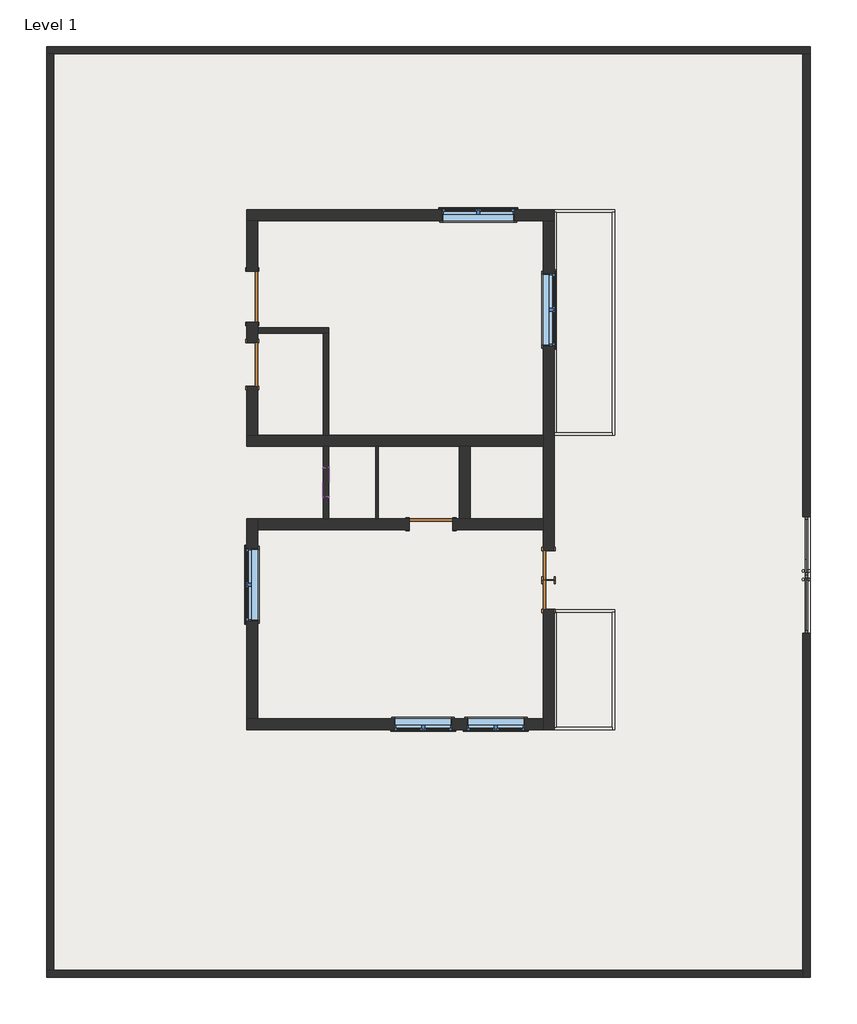
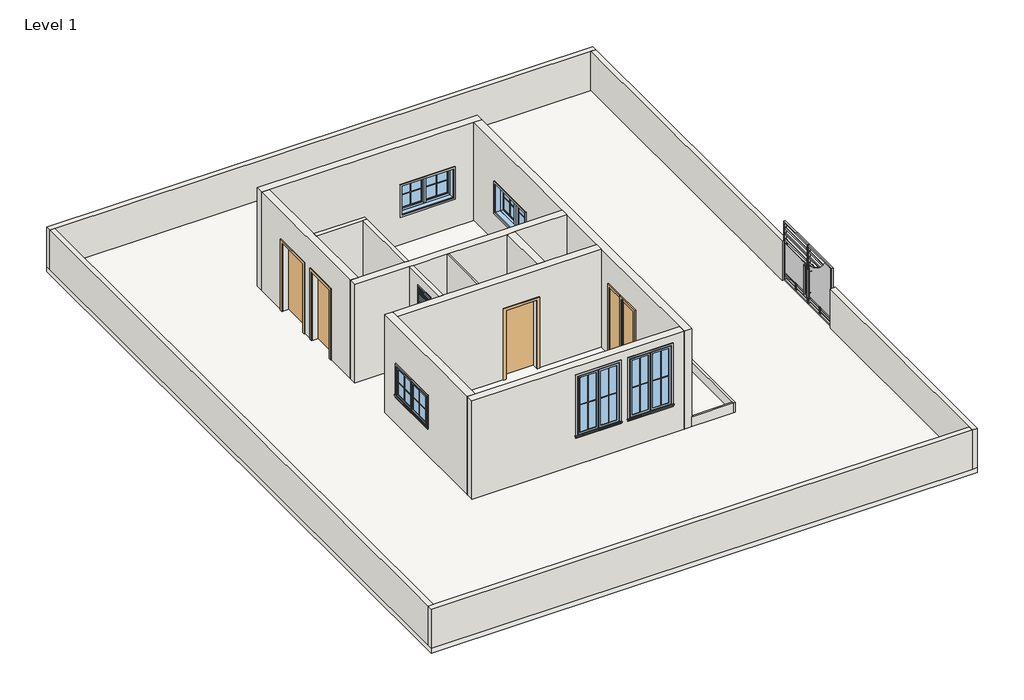
# One storey: 25 walls, 21 proxies, 6 windows, 5 doors, 1 slab.
"""IFC4 building model written with IfcOpenShell, lengths in millimetres."""

from ifc_helpers import new_model, si_unit, frame, origin, origin_with_axes, place, context, project, spatial, polyline, outline, extrude, faceted_brep, transform, mapped, element, save
from components import generic_models_113f6068, muntin_pattern_2x2_muntin_pattern_2x2_9352d081, muntin_pattern_2x2_muntin_pattern_2x2_5c2cbe28, muntin_pattern_2x2_muntin_pattern_2x2_2b4d9f72, muntin_pattern_2x2_muntin_pattern_2x2_ef995ed3, trim_window_exterior_flat_with_sill_979bde60, trim_window_exterior_flat_with_sill_b7e4d11c, trim_window_interior_flat_picture_frame_7883d11b, trim_window_interior_flat_picture_frame_936b8d2a, single_flush_door_2_0d3b4037, single_flush_door_2_4a3212df, door_a90ba1ad, door_0ca8825f, door_9d399b00, window_casement_double_c1d95f0f, window_casement_double_wall_4_6ca1769e, window_d39e7ecb

model = new_model("IFC4")

# Units and contexts
model_context = context("Model", 3, world=origin())
ifc_project = project(units=[si_unit("LENGTHUNIT", "METRE", prefix="MILLI")], contexts=[model_context])

# Site, building, storey
site = spatial("IfcSite", under=ifc_project)
building = spatial("IfcBuilding", under=site)
storey = spatial("IfcBuildingStorey", under=building, Name="Level 1", Elevation=0.0)

# Proxies
placement = place(None, origin())
generic_models_shape = generic_models_113f6068(model_context)
element("IfcBuildingElementProxy", 1, Name="Generic Models", at=placement, inside=storey, context=model_context, shape_type="MappedRepresentation", body=[
    mapped(generic_models_shape, transform((6909.9576308, -2125.2492544, 0.0), x_axis=(0.0, 1.0, 0.0), y_axis=(-1.0, 0.0, 0.0), z_axis=(0.0, 0.0, 1.0))),
])
muntin_pattern_2x2_muntin_pattern_2x2_shape = muntin_pattern_2x2_muntin_pattern_2x2_9352d081(model_context)
element("IfcBuildingElementProxy", 2, Name="Muntin Pattern_2x2 : Muntin Pattern_2x2", ObjectType="Muntin Pattern_2x2 : Muntin Pattern_2x2", at=placement, inside=storey, context=model_context, shape_type="MappedRepresentation", body=[
    mapped(muntin_pattern_2x2_muntin_pattern_2x2_shape, transform((-4785.3510342, -2707.8617544, 984.25), x_axis=(0.0, 1.0, 0.0), y_axis=(-1.0, 0.0, 0.0), z_axis=(0.0, 0.0, 1.0))),
])
element("IfcBuildingElementProxy", 3, Name="Muntin Pattern_2x2 : Muntin Pattern_2x2", ObjectType="Muntin Pattern_2x2 : Muntin Pattern_2x2", at=placement, inside=storey, context=model_context, shape_type="MappedRepresentation", body=[
    mapped(muntin_pattern_2x2_muntin_pattern_2x2_shape, transform((1634.4989658, 3816.7632456, 984.25), x_axis=(0.0, -1.0, 0.0), y_axis=(1.0, 0.0, 0.0), z_axis=(0.0, 0.0, 1.0))),
])
element("IfcBuildingElementProxy", 4, Name="Muntin Pattern_2x2 : Muntin Pattern_2x2", ObjectType="Muntin Pattern_2x2 : Muntin Pattern_2x2", at=placement, inside=storey, context=model_context, shape_type="MappedRepresentation", body=[
    mapped(muntin_pattern_2x2_muntin_pattern_2x2_shape, transform((-322.8885342, 5523.3257456, 984.25), x_axis=(1.0, 0.0, 0.0), y_axis=(0.0, 1.0, 0.0), z_axis=(0.0, 0.0, 1.0))),
])
muntin_pattern_2x2_muntin_pattern_2x2_2_shape = muntin_pattern_2x2_muntin_pattern_2x2_5c2cbe28(model_context)
element("IfcBuildingElementProxy", 5, Name="Muntin Pattern_2x2 : Muntin Pattern_2x2", ObjectType="Muntin Pattern_2x2 : Muntin Pattern_2x2", at=placement, inside=storey, context=model_context, shape_type="MappedRepresentation", body=[
    mapped(muntin_pattern_2x2_muntin_pattern_2x2_2_shape, transform((-4785.3510342, -1949.0367544, 984.25), x_axis=(0.0, -1.0, 0.0), y_axis=(1.0, 0.0, 0.0), z_axis=(0.0, 0.0, 1.0))),
])
element("IfcBuildingElementProxy", 6, Name="Muntin Pattern_2x2 : Muntin Pattern_2x2", ObjectType="Muntin Pattern_2x2 : Muntin Pattern_2x2", at=placement, inside=storey, context=model_context, shape_type="MappedRepresentation", body=[
    mapped(muntin_pattern_2x2_muntin_pattern_2x2_2_shape, transform((1634.4989658, 3057.9382456, 984.25), x_axis=(0.0, 1.0, 0.0), y_axis=(-1.0, 0.0, 0.0), z_axis=(0.0, 0.0, 1.0))),
])
element("IfcBuildingElementProxy", 7, Name="Muntin Pattern_2x2 : Muntin Pattern_2x2", ObjectType="Muntin Pattern_2x2 : Muntin Pattern_2x2", at=placement, inside=storey, context=model_context, shape_type="MappedRepresentation", body=[
    mapped(muntin_pattern_2x2_muntin_pattern_2x2_2_shape, transform((435.9364658, 5523.3257456, 984.25), x_axis=(-1.0, 0.0, 0.0), y_axis=(0.0, -1.0, 0.0), z_axis=(0.0, 0.0, 1.0))),
])
muntin_pattern_2x2_muntin_pattern_2x2_3_shape = muntin_pattern_2x2_muntin_pattern_2x2_2b4d9f72(model_context)
element("IfcBuildingElementProxy", 8, Name="Muntin Pattern_2x2 : Muntin Pattern_2x2", ObjectType="Muntin Pattern_2x2 : Muntin Pattern_2x2", at=placement, inside=storey, context=model_context, shape_type="MappedRepresentation", body=[
    mapped(muntin_pattern_2x2_muntin_pattern_2x2_3_shape, transform((-795.9635342, -5354.2242544, 984.25), x_axis=(-1.0, 0.0, 0.0), y_axis=(0.0, -1.0, 0.0), z_axis=(0.0, 0.0, 1.0))),
])
element("IfcBuildingElementProxy", 9, Name="Muntin Pattern_2x2 : Muntin Pattern_2x2", ObjectType="Muntin Pattern_2x2 : Muntin Pattern_2x2", at=placement, inside=storey, context=model_context, shape_type="MappedRepresentation", body=[
    mapped(muntin_pattern_2x2_muntin_pattern_2x2_3_shape, transform((728.0364658, -5354.2242544, 984.25), x_axis=(-1.0, 0.0, 0.0), y_axis=(0.0, -1.0, 0.0), z_axis=(0.0, 0.0, 1.0))),
])
muntin_pattern_2x2_muntin_pattern_2x2_4_shape = muntin_pattern_2x2_muntin_pattern_2x2_ef995ed3(model_context)
element("IfcBuildingElementProxy", 10, Name="Muntin Pattern_2x2 : Muntin Pattern_2x2", ObjectType="Muntin Pattern_2x2 : Muntin Pattern_2x2", at=placement, inside=storey, context=model_context, shape_type="MappedRepresentation", body=[
    mapped(muntin_pattern_2x2_muntin_pattern_2x2_4_shape, transform((-1402.3885342, -5354.2242544, 984.25), x_axis=(1.0, 0.0, 0.0), y_axis=(0.0, 1.0, 0.0), z_axis=(0.0, 0.0, 1.0))),
])
element("IfcBuildingElementProxy", 11, Name="Muntin Pattern_2x2 : Muntin Pattern_2x2", ObjectType="Muntin Pattern_2x2 : Muntin Pattern_2x2", at=placement, inside=storey, context=model_context, shape_type="MappedRepresentation", body=[
    mapped(muntin_pattern_2x2_muntin_pattern_2x2_4_shape, transform((121.6114658, -5354.2242544, 984.25), x_axis=(1.0, 0.0, 0.0), y_axis=(0.0, 1.0, 0.0), z_axis=(0.0, 0.0, 1.0))),
])
trim_window_exterior_flat_with_sill_shape = trim_window_exterior_flat_with_sill_979bde60(model_context)
element("IfcBuildingElementProxy", 12, Name="Trim-Window-Exterior-Flat : with Sill", ObjectType="Trim-Window-Exterior-Flat : with Sill", at=placement, inside=storey, context=model_context, shape_type="MappedRepresentation", body=[
    mapped(trim_window_exterior_flat_with_sill_shape, transform((-4794.8760342, -2328.4492544, 1828.8), x_axis=(0.0, -1.0, 0.0), y_axis=(0.0, 0.0, 1.0), z_axis=(-1.0, 0.0, 0.0))),
])
element("IfcBuildingElementProxy", 13, Name="Trim-Window-Exterior-Flat : with Sill", ObjectType="Trim-Window-Exterior-Flat : with Sill", at=placement, inside=storey, context=model_context, shape_type="MappedRepresentation", body=[
    mapped(trim_window_exterior_flat_with_sill_shape, transform((1644.0239658, 3437.3507456, 1828.8), x_axis=(0.0, 1.0, 0.0), y_axis=(0.0, 0.0, 1.0), z_axis=(1.0, 0.0, 0.0))),
])
element("IfcBuildingElementProxy", 14, Name="Trim-Window-Exterior-Flat : with Sill", ObjectType="Trim-Window-Exterior-Flat : with Sill", at=placement, inside=storey, context=model_context, shape_type="MappedRepresentation", body=[
    mapped(trim_window_exterior_flat_with_sill_shape, transform((56.5239658, 5532.8507456, 1828.8), x_axis=(-1.0, 0.0, 0.0), y_axis=(0.0, 0.0, 1.0), z_axis=(0.0, 1.0, 0.0))),
])
trim_window_exterior_flat_with_sill_2_shape = trim_window_exterior_flat_with_sill_b7e4d11c(model_context)
element("IfcBuildingElementProxy", 15, Name="Trim-Window-Exterior-Flat : with Sill", ObjectType="Trim-Window-Exterior-Flat : with Sill", at=placement, inside=storey, context=model_context, shape_type="MappedRepresentation", body=[
    mapped(trim_window_exterior_flat_with_sill_2_shape, transform((-1099.1760342, -5363.7492544, 2743.2), x_axis=(1.0, 0.0, 0.0), y_axis=(0.0, 0.0, 1.0), z_axis=(0.0, -1.0, 0.0))),
])
element("IfcBuildingElementProxy", 16, Name="Trim-Window-Exterior-Flat : with Sill", ObjectType="Trim-Window-Exterior-Flat : with Sill", at=placement, inside=storey, context=model_context, shape_type="MappedRepresentation", body=[
    mapped(trim_window_exterior_flat_with_sill_2_shape, transform((424.8239658, -5363.7492544, 2743.2), x_axis=(1.0, 0.0, 0.0), y_axis=(0.0, 0.0, 1.0), z_axis=(0.0, -1.0, 0.0))),
])
trim_window_interior_flat_picture_frame_shape = trim_window_interior_flat_picture_frame_7883d11b(model_context)
element("IfcBuildingElementProxy", 17, Name="Trim-Window-Interior-Flat : Picture Frame", ObjectType="Trim-Window-Interior-Flat : Picture Frame", at=placement, inside=storey, context=model_context, shape_type="MappedRepresentation", body=[
    mapped(trim_window_interior_flat_picture_frame_shape, transform((-4566.2760342, -2328.4492544, 1828.8), x_axis=(0.0, 1.0, 0.0), y_axis=(0.0, 0.0, 1.0), z_axis=(1.0, 0.0, 0.0))),
])
element("IfcBuildingElementProxy", 18, Name="Trim-Window-Interior-Flat : Picture Frame", ObjectType="Trim-Window-Interior-Flat : Picture Frame", at=placement, inside=storey, context=model_context, shape_type="MappedRepresentation", body=[
    mapped(trim_window_interior_flat_picture_frame_shape, transform((1415.4239658, 3437.3507456, 1828.8), x_axis=(0.0, -1.0, 0.0), y_axis=(0.0, 0.0, 1.0), z_axis=(-1.0, 0.0, 0.0))),
])
element("IfcBuildingElementProxy", 19, Name="Trim-Window-Interior-Flat : Picture Frame", ObjectType="Trim-Window-Interior-Flat : Picture Frame", at=placement, inside=storey, context=model_context, shape_type="MappedRepresentation", body=[
    mapped(trim_window_interior_flat_picture_frame_shape, transform((56.5239658, 5304.2507456, 1828.8), x_axis=(1.0, 0.0, 0.0), y_axis=(0.0, 0.0, 1.0), z_axis=(0.0, -1.0, 0.0))),
])
trim_window_interior_flat_picture_frame_2_shape = trim_window_interior_flat_picture_frame_936b8d2a(model_context)
element("IfcBuildingElementProxy", 20, Name="Trim-Window-Interior-Flat : Picture Frame", ObjectType="Trim-Window-Interior-Flat : Picture Frame", at=placement, inside=storey, context=model_context, shape_type="MappedRepresentation", body=[
    mapped(trim_window_interior_flat_picture_frame_2_shape, transform((-1099.1760342, -5135.1492544, 2743.2), x_axis=(-1.0, 0.0, 0.0), y_axis=(0.0, 0.0, 1.0), z_axis=(0.0, 1.0, 0.0))),
])
element("IfcBuildingElementProxy", 21, Name="Trim-Window-Interior-Flat : Picture Frame", ObjectType="Trim-Window-Interior-Flat : Picture Frame", at=placement, inside=storey, context=model_context, shape_type="MappedRepresentation", body=[
    mapped(trim_window_interior_flat_picture_frame_2_shape, transform((424.8239658, -5135.1492544, 2743.2), x_axis=(-1.0, 0.0, 0.0), y_axis=(0.0, 0.0, 1.0), z_axis=(0.0, 1.0, 0.0))),
])

# Doors
single_flush_door_2_shape = single_flush_door_2_0d3b4037(model_context)
element("IfcDoor", 22, ObjectType="Single-Flush : door 2'", at=placement, inside=storey, context=model_context, shape_type="MappedRepresentation", body=[
    mapped(single_flush_door_2_shape, transform((1529.7239658, -1922.0492544, 0.0), x_axis=(0.0, 1.0, 0.0), y_axis=(-1.0, 0.0, 0.0), z_axis=(0.0, 0.0, 1.0))),
])
single_flush_door_2_2_shape = single_flush_door_2_4a3212df(model_context)
element("IfcDoor", 23, ObjectType="Single-Flush : door 2'", at=placement, inside=storey, context=model_context, shape_type="MappedRepresentation", body=[
    mapped(single_flush_door_2_2_shape, transform((1529.7239658, -2537.9992544, 0.0), x_axis=(0.0, -1.0, 0.0), y_axis=(1.0, 0.0, 0.0), z_axis=(0.0, 0.0, 1.0))),
])
door_shape = door_a90ba1ad(model_context)
element("IfcDoor", 24, ObjectType="Single-Flush : door 2'6\"", at=placement, inside=storey, context=model_context, shape_type="MappedRepresentation", body=[
    mapped(door_shape, transform((-4680.5760342, 2288.0007456, 0.0), x_axis=(0.0, 1.0, 0.0), y_axis=(-1.0, 0.0, 0.0), z_axis=(0.0, 0.0, 1.0))),
])
door_2_shape = door_0ca8825f(model_context)
element("IfcDoor", 25, ObjectType="Single-Flush : door 2'6\"", at=placement, inside=storey, context=model_context, shape_type="MappedRepresentation", body=[
    mapped(door_2_shape, transform((-934.0760342, -1058.4492544, 0.0), x_axis=(1.0, 0.0, 0.0), y_axis=(0.0, 1.0, 0.0), z_axis=(0.0, 0.0, 1.0))),
])
door_3_shape = door_9d399b00(model_context)
element("IfcDoor", 26, ObjectType="Single-Flush : door 3'6\"", at=placement, inside=storey, context=model_context, shape_type="MappedRepresentation", body=[
    mapped(door_3_shape, transform((-4680.5760342, 3710.4007456, 0.0), x_axis=(0.0, -1.0, 0.0), y_axis=(1.0, 0.0, 0.0), z_axis=(0.0, 0.0, 1.0))),
])

# Slab
element("IfcSlab", 27, ObjectType="floor 6\"", at=placement, inside=storey, context=model_context, shape_type="SweptSolid", body=[
    extrude(outline(polyline([(7011.5576308, 8950.777895), (7011.5576308, -10556.422105), (-8990.4423692, -10556.422105), (-8990.4423692, 8950.777895), (7011.5576308, 8950.777895)])), frame((0.0, 0.0, -152.4), z_axis=(0.0, 0.0, 1.0), x_axis=(1.0, 0.0, 0.0)), (0.0, 0.0, 1.0), 152.4),
])

# Walls
element("IfcWall", 28, at=placement, inside=storey, context=model_context, shape_type="Brep", body=[
    faceted_brep([(-8990.4423692, 8798.377895, 0.0), (-8838.0423692, 8798.377895, 0.0), (6859.1576308, 8798.377895, 0.0), (7011.5576308, 8798.377895, 0.0), (7011.5576308, 8798.377895, 1219.2), (6859.1576308, 8798.377895, 1219.2), (-8838.0423692, 8798.377895, 1219.2), (-8990.4423692, 8798.377895, 1219.2), (-8990.4423692, 8950.777895, 0.0), (-8990.4423692, 8950.777895, 1219.2), (7011.5576308, 8950.777895, 1219.2), (7011.5576308, 8950.777895, 0.0)], [[[0, 1, 2, 3, 4, 5, 6, 7]], [[8, 9, 10, 11]], [[3, 2, 1, 0, 8, 11]], [[7, 6, 5, 4, 10, 9]], [[4, 3, 11, 10]], [[0, 7, 9, 8]]]),
])
element("IfcWall", 29, at=placement, inside=storey, context=model_context, shape_type="SweptSolid", body=[
    extrude(outline(polyline([(6859.1576308, -906.0492544), (6859.1576308, 8798.377895), (7011.5576308, 8798.377895), (7011.5576308, -906.0492544), (6859.1576308, -906.0492544)])), origin_with_axes(), (0.0, 0.0, 1.0), 1219.2),
])
element("IfcWall", 30, at=placement, inside=storey, context=model_context, shape_type="Brep", body=[
    faceted_brep([(6859.1576308, -10404.022105, 0.0), (-8838.0423692, -10404.022105, 0.0), (-8990.4423692, -10404.022105, 0.0), (-8990.4423692, -10404.022105, 1219.2), (-8838.0423692, -10404.022105, 1219.2), (6859.1576308, -10404.022105, 1219.2), (6859.1576308, -10556.422105, 0.0), (6859.1576308, -10556.422105, 1219.2), (-8990.4423692, -10556.422105, 1219.2), (-8990.4423692, -10556.422105, 0.0)], [[[0, 1, 2, 3, 4, 5]], [[6, 7, 8, 9]], [[2, 1, 0, 6, 9]], [[5, 4, 3, 8, 7]], [[0, 5, 7, 6]], [[3, 2, 9, 8]]]),
])
element("IfcWall", 31, at=placement, inside=storey, context=model_context, shape_type="SweptSolid", body=[
    extrude(outline(polyline([(-8838.0423692, 8798.377895), (-8838.0423692, -10404.022105), (-8990.4423692, -10404.022105), (-8990.4423692, 8798.377895), (-8838.0423692, 8798.377895)])), origin_with_axes(), (0.0, 0.0, 1.0), 1219.2),
])
element("IfcWall", 32, at=placement, inside=storey, context=model_context, shape_type="Brep", body=[
    faceted_brep([(6859.1576308, -3344.4492544, 0.0), (6859.1576308, -10404.022105, 0.0), (6859.1576308, -10556.422105, 0.0), (6859.1576308, -10556.422105, 1219.2), (6859.1576308, -10404.022105, 1219.2), (6859.1576308, -3344.4492544, 1219.2), (7011.5576308, -3344.4492544, 0.0), (7011.5576308, -3344.4492544, 1219.2), (7011.5576308, -10556.422105, 1219.2), (7011.5576308, -10556.422105, 0.0)], [[[0, 1, 2, 3, 4, 5]], [[6, 7, 8, 9]], [[2, 1, 0, 6, 9]], [[5, 4, 3, 8, 7]], [[0, 5, 7, 6]], [[3, 2, 9, 8]]]),
])
element("IfcWall", 33, ObjectType="wall 2\"", at=placement, inside=storey, context=model_context, shape_type="SweptSolid", body=[
    extrude(outline(polyline([(-2089.7760342, -944.1492544), (-2089.7760342, 579.8507456), (-2038.9760342, 579.8507456), (-2038.9760342, -944.1492544), (-2089.7760342, -944.1492544)])), origin_with_axes(), (0.0, 0.0, 1.0), 3048.0),
])
element("IfcWall", 34, ObjectType="wall 2\"", at=placement, inside=storey, context=model_context, shape_type="Brep", body=[
    faceted_brep([(1644.0239658, 5482.0507456, 0.0), (1694.8239658, 5482.0507456, 0.0), (2863.2239658, 5482.0507456, 0.0), (2914.0239658, 5482.0507456, 0.0), (2914.0239658, 5482.0507456, 304.8), (2863.2239658, 5482.0507456, 304.8), (1694.8239658, 5482.0507456, 304.8), (1644.0239658, 5482.0507456, 304.8), (1644.0239658, 5532.8507456, 0.0), (1644.0239658, 5532.8507456, 304.8), (2914.0239658, 5532.8507456, 304.8), (2914.0239658, 5532.8507456, 0.0)], [[[0, 1, 2, 3, 4, 5, 6, 7]], [[8, 9, 10, 11]], [[3, 2, 1, 0, 8, 11]], [[7, 6, 5, 4, 10, 9]], [[0, 7, 9, 8]], [[4, 3, 11, 10]]]),
])
element("IfcWall", 35, ObjectType="wall 2\"", at=placement, inside=storey, context=model_context, shape_type="Brep", body=[
    faceted_brep([(2863.2239658, 5482.0507456, 0.0), (2863.2239658, 859.2507456, 0.0), (2863.2239658, 808.4507456, 0.0), (2863.2239658, 808.4507456, 304.8), (2863.2239658, 859.2507456, 304.8), (2863.2239658, 5482.0507456, 304.8), (2914.0239658, 5482.0507456, 0.0), (2914.0239658, 5482.0507456, 304.8), (2914.0239658, 808.4507456, 304.8), (2914.0239658, 808.4507456, 0.0)], [[[0, 1, 2, 3, 4, 5]], [[6, 7, 8, 9]], [[2, 1, 0, 6, 9]], [[5, 4, 3, 8, 7]], [[0, 5, 7, 6]], [[3, 2, 9, 8]]]),
])
element("IfcWall", 36, ObjectType="wall 2\"", at=placement, inside=storey, context=model_context, shape_type="Brep", body=[
    faceted_brep([(2863.2239658, 859.2507456, 0.0), (1694.8239658, 859.2507456, 0.0), (1644.0239658, 859.2507456, 0.0), (1644.0239658, 859.2507456, 304.8), (1694.8239658, 859.2507456, 304.8), (2863.2239658, 859.2507456, 304.8), (2863.2239658, 808.4507456, 0.0), (2863.2239658, 808.4507456, 304.8), (1644.0239658, 808.4507456, 304.8), (1644.0239658, 808.4507456, 0.0)], [[[0, 1, 2, 3, 4, 5]], [[6, 7, 8, 9]], [[2, 1, 0, 6, 9]], [[5, 4, 3, 8, 7]], [[0, 5, 7, 6]], [[3, 2, 9, 8]]]),
])
element("IfcWall", 37, ObjectType="wall 2\"", at=placement, inside=storey, context=model_context, shape_type="Brep", body=[
    faceted_brep([(1694.8239658, 859.2507456, 0.0), (1694.8239658, 5482.0507456, 0.0), (1694.8239658, 5482.0507456, 304.8), (1694.8239658, 859.2507456, 304.8), (1644.0239658, 859.2507456, 0.0), (1644.0239658, 859.2507456, 304.8), (1644.0239658, 5482.0507456, 304.8), (1644.0239658, 5482.0507456, 0.0), (1644.0239658, 5304.2507456, 0.0)], [[[0, 1, 2, 3]], [[4, 5, 6, 7, 8]], [[1, 0, 4, 8, 7]], [[3, 2, 6, 5]], [[2, 1, 7, 6]], [[0, 3, 5, 4]]]),
])
element("IfcWall", 38, ObjectType="wall 2\"", at=placement, inside=storey, context=model_context, shape_type="Brep", body=[
    faceted_brep([(1644.0239658, -2899.9492544, 0.0), (1694.8239658, -2899.9492544, 0.0), (2863.2239658, -2899.9492544, 0.0), (2914.0239658, -2899.9492544, 0.0), (2914.0239658, -2899.9492544, 304.8), (2863.2239658, -2899.9492544, 304.8), (1694.8239658, -2899.9492544, 304.8), (1644.0239658, -2899.9492544, 304.8), (1644.0239658, -2849.1492544, 0.0), (1644.0239658, -2849.1492544, 304.8), (2914.0239658, -2849.1492544, 304.8), (2914.0239658, -2849.1492544, 0.0)], [[[0, 1, 2, 3, 4, 5, 6, 7]], [[8, 9, 10, 11]], [[3, 2, 1, 0, 8, 11]], [[7, 6, 5, 4, 10, 9]], [[0, 7, 9, 8]], [[4, 3, 11, 10]]]),
])
element("IfcWall", 39, ObjectType="wall 2\"", at=placement, inside=storey, context=model_context, shape_type="Brep", body=[
    faceted_brep([(2863.2239658, -2899.9492544, 0.0), (2863.2239658, -5312.9492544, 0.0), (2863.2239658, -5363.7492544, 0.0), (2863.2239658, -5363.7492544, 304.8), (2863.2239658, -5312.9492544, 304.8), (2863.2239658, -2899.9492544, 304.8), (2914.0239658, -2899.9492544, 0.0), (2914.0239658, -2899.9492544, 304.8), (2914.0239658, -5363.7492544, 304.8), (2914.0239658, -5363.7492544, 0.0)], [[[0, 1, 2, 3, 4, 5]], [[6, 7, 8, 9]], [[2, 1, 0, 6, 9]], [[5, 4, 3, 8, 7]], [[0, 5, 7, 6]], [[3, 2, 9, 8]]]),
])
element("IfcWall", 40, ObjectType="wall 2\"", at=placement, inside=storey, context=model_context, shape_type="Brep", body=[
    faceted_brep([(2863.2239658, -5312.9492544, 0.0), (1694.8239658, -5312.9492544, 0.0), (1644.0239658, -5312.9492544, 0.0), (1644.0239658, -5312.9492544, 304.8), (1694.8239658, -5312.9492544, 304.8), (2863.2239658, -5312.9492544, 304.8), (2863.2239658, -5363.7492544, 0.0), (2863.2239658, -5363.7492544, 304.8), (1644.0239658, -5363.7492544, 304.8), (1644.0239658, -5363.7492544, 0.0)], [[[0, 1, 2, 3, 4, 5]], [[6, 7, 8, 9]], [[2, 1, 0, 6, 9]], [[5, 4, 3, 8, 7]], [[0, 5, 7, 6]], [[3, 2, 9, 8]]]),
])
element("IfcWall", 41, ObjectType="wall 2\"", at=placement, inside=storey, context=model_context, shape_type="SweptSolid", body=[
    extrude(outline(polyline([(1694.8239658, -2899.9492544), (1694.8239658, -5312.9492544), (1644.0239658, -5312.9492544), (1644.0239658, -2899.9492544), (1694.8239658, -2899.9492544)])), origin_with_axes(), (0.0, 0.0, 1.0), 304.8),
])
element("IfcWall", 42, ObjectType="wall 4.5\"", at=placement, inside=storey, context=model_context, shape_type="Brep", body=[
    faceted_brep([(-4566.2760342, 2942.0507456, 0.0), (-3194.6760342, 2942.0507456, 0.0), (-3080.3760342, 2942.0507456, 0.0), (-3080.3760342, 2942.0507456, 3048.0), (-3194.6760342, 2942.0507456, 3048.0), (-4566.2760342, 2942.0507456, 3048.0), (-4566.2760342, 3056.3507456, 0.0), (-4566.2760342, 3056.3507456, 3048.0), (-3080.3760342, 3056.3507456, 3048.0), (-3080.3760342, 3056.3507456, 0.0)], [[[0, 1, 2, 3, 4, 5]], [[6, 7, 8, 9]], [[2, 1, 0, 6, 9]], [[0, 5, 7, 6]], [[3, 2, 9, 8]], [[5, 4, 3, 8, 7]]]),
])
element("IfcWall", 43, ObjectType="wall 4.5\"", at=placement, inside=storey, context=model_context, shape_type="SweptSolid", body=[
    extrude(outline(polyline([(-3194.6760342, 808.4507456), (-3194.6760342, 2942.0507456), (-3080.3760342, 2942.0507456), (-3080.3760342, 808.4507456), (-3194.6760342, 808.4507456)])), origin_with_axes(), (0.0, 0.0, 1.0), 3048.0),
])
element("IfcWall", 44, ObjectType="wall 4.5\"", at=placement, inside=storey, context=model_context, shape_type="SweptSolid", body=[
    extrude(outline(polyline([(579.8507456, 0.0), (-944.1492544, 0.0), (-944.1492544, 3048.0), (579.8507456, 3048.0), (579.8507456, 0.0)]), holes=[polyline([(-486.9492544, 2743.2), (-486.9492544, 2133.6), (122.6507456, 2133.6), (122.6507456, 2743.2), (-486.9492544, 2743.2)])]), frame((-3194.6760342, 0.0, 0.0), z_axis=(1.0, 0.0, 0.0), x_axis=(0.0, 1.0, 0.0)), (0.0, 0.0, 1.0), 114.3),
])
element("IfcWall", 45, ObjectType="wall 9\"", at=placement, inside=storey, context=model_context, shape_type="Brep", body=[
    faceted_brep([(-4794.8760342, 5304.2507456, 0.0), (-4566.2760342, 5304.2507456, 0.0), (1415.4239658, 5304.2507456, 0.0), (1644.0239658, 5304.2507456, 0.0), (1644.0239658, 5304.2507456, 3048.0), (1415.4239658, 5304.2507456, 3048.0), (-4566.2760342, 5304.2507456, 3048.0), (-4794.8760342, 5304.2507456, 3048.0), (818.5239658, 5304.2507456, 1828.8), (818.5239658, 5304.2507456, 914.4), (-705.4760342, 5304.2507456, 914.4), (-705.4760342, 5304.2507456, 1828.8), (-4794.8760342, 5532.8507456, 0.0), (-4794.8760342, 5532.8507456, 3048.0), (1644.0239658, 5532.8507456, 3048.0), (1644.0239658, 5532.8507456, 304.8), (1644.0239658, 5532.8507456, 0.0), (818.5239658, 5532.8507456, 1828.8), (-705.4760342, 5532.8507456, 1828.8), (-705.4760342, 5532.8507456, 914.4), (818.5239658, 5532.8507456, 914.4), (1644.0239658, 5482.0507456, 0.0)], [[[0, 1, 2, 3, 4, 5, 6, 7], [8, 9, 10, 11]], [[12, 13, 14, 15, 16], [17, 18, 19, 20]], [[3, 2, 1, 0, 12, 16, 21]], [[0, 7, 13, 12]], [[3, 21, 16, 15, 14, 4]], [[9, 8, 17, 20]], [[10, 9, 20, 19]], [[11, 10, 19, 18]], [[8, 11, 18, 17]], [[7, 6, 5, 4, 14, 13]]]),
])
element("IfcWall", 46, ObjectType="wall 9\"", at=placement, inside=storey, context=model_context, shape_type="Brep", body=[
    faceted_brep([(1415.4239658, 5304.2507456, 3048.0), (1415.4239658, 5304.2507456, 0.0), (1415.4239658, 808.4507456, 0.0), (1415.4239658, 579.8507456, 0.0), (1415.4239658, -944.1492544, 0.0), (1415.4239658, -1172.7492544, 0.0), (1415.4239658, -1617.2492544, 0.0), (1415.4239658, -1617.2492544, 2133.6), (1415.4239658, -2226.8492544, 2133.6), (1415.4239658, -2226.8492544, 0.0), (1415.4239658, -2233.1992544, 0.0), (1415.4239658, -2233.1992544, 2133.6), (1415.4239658, -2842.7992544, 2133.6), (1415.4239658, -2842.7992544, 0.0), (1415.4239658, -5135.1492544, 0.0), (1415.4239658, -5363.7492544, 0.0), (1415.4239658, -5363.7492544, 3048.0), (1415.4239658, -5135.1492544, 3048.0), (1415.4239658, -1172.7492544, 3048.0), (1415.4239658, -944.1492544, 3048.0), (1415.4239658, 579.8507456, 3048.0), (1415.4239658, 808.4507456, 3048.0), (1415.4239658, 2675.3507456, 1828.8), (1415.4239658, 2675.3507456, 914.4), (1415.4239658, 4199.3507456, 914.4), (1415.4239658, 4199.3507456, 1828.8), (1644.0239658, 5304.2507456, 0.0), (1644.0239658, 5304.2507456, 3048.0), (1644.0239658, -5363.7492544, 3048.0), (1644.0239658, -5363.7492544, 304.8), (1644.0239658, -5363.7492544, 0.0), (1644.0239658, -5312.9492544, 0.0), (1644.0239658, -2899.9492544, 0.0), (1644.0239658, -2849.1492544, 0.0), (1644.0239658, -2842.7992544, 0.0), (1644.0239658, -2842.7992544, 2133.6), (1644.0239658, -2233.1992544, 2133.6), (1644.0239658, -2233.1992544, 0.0), (1644.0239658, -2226.8492544, 0.0), (1644.0239658, -2226.8492544, 2133.6), (1644.0239658, -1617.2492544, 2133.6), (1644.0239658, -1617.2492544, 0.0), (1644.0239658, 808.4507456, 0.0), (1644.0239658, 859.2507456, 0.0), (1644.0239658, 2675.3507456, 1828.8), (1644.0239658, 4199.3507456, 1828.8), (1644.0239658, 4199.3507456, 914.4), (1644.0239658, 2675.3507456, 914.4)], [[[0, 1, 2, 3, 4, 5, 6, 7, 8, 9, 10, 11, 12, 13, 14, 15, 16, 17, 18, 19, 20, 21], [22, 23, 24, 25]], [[26, 27, 28, 29, 30, 31, 32, 33, 34, 35, 36, 37, 38, 39, 40, 41, 42, 43], [44, 45, 46, 47]], [[1, 26, 43, 42, 41, 6, 5, 4, 3, 2]], [[30, 15, 14, 13, 34, 33, 32, 31]], [[9, 38, 37, 10]], [[26, 1, 0, 27]], [[15, 30, 29, 28, 16]], [[23, 22, 44, 47]], [[24, 23, 47, 46]], [[25, 24, 46, 45]], [[22, 25, 45, 44]], [[7, 6, 41, 40]], [[8, 7, 40, 39]], [[9, 8, 39, 38]], [[12, 35, 34, 13]], [[35, 12, 11, 36]], [[36, 11, 10, 37]], [[0, 21, 20, 19, 18, 17, 16, 28, 27]]]),
])
element("IfcWall", 47, ObjectType="wall 9\"", at=placement, inside=storey, context=model_context, shape_type="Brep", body=[
    faceted_brep([(1415.4239658, 808.4507456, 0.0), (-3080.3760342, 808.4507456, 0.0), (-3194.6760342, 808.4507456, 0.0), (-4566.2760342, 808.4507456, 0.0), (-4794.8760342, 808.4507456, 0.0), (-4794.8760342, 808.4507456, 3048.0), (-4566.2760342, 808.4507456, 3048.0), (-3194.6760342, 808.4507456, 3048.0), (-3080.3760342, 808.4507456, 3048.0), (1415.4239658, 808.4507456, 3048.0), (1415.4239658, 579.8507456, 0.0), (1415.4239658, 579.8507456, 3048.0), (-108.5760342, 579.8507456, 3048.0), (-337.1760342, 579.8507456, 3048.0), (-2038.9760342, 579.8507456, 3048.0), (-2089.7760342, 579.8507456, 3048.0), (-3080.3760342, 579.8507456, 3048.0), (-3194.6760342, 579.8507456, 3048.0), (-4794.8760342, 579.8507456, 3048.0), (-4794.8760342, 579.8507456, 0.0), (-3194.6760342, 579.8507456, 0.0), (-3080.3760342, 579.8507456, 0.0), (-2089.7760342, 579.8507456, 0.0), (-2038.9760342, 579.8507456, 0.0), (-337.1760342, 579.8507456, 0.0), (-108.5760342, 579.8507456, 0.0)], [[[0, 1, 2, 3, 4, 5, 6, 7, 8, 9]], [[10, 11, 12, 13, 14, 15, 16, 17, 18, 19, 20, 21, 22, 23, 24, 25]], [[4, 3, 2, 1, 0, 10, 25, 24, 23, 22, 21, 20, 19]], [[0, 9, 11, 10]], [[5, 4, 19, 18]], [[9, 8, 7, 6, 5, 18, 17, 16, 15, 14, 13, 12, 11]]]),
])
element("IfcWall", 48, ObjectType="wall 9\"", at=placement, inside=storey, context=model_context, shape_type="Brep", body=[
    faceted_brep([(-4566.2760342, 2745.2007456, 2133.6), (-4566.2760342, 2745.2007456, 0.0), (-4566.2760342, 2942.0507456, 0.0), (-4566.2760342, 3056.3507456, 0.0), (-4566.2760342, 3177.0007456, 0.0), (-4566.2760342, 3177.0007456, 2133.6), (-4566.2760342, 4243.8007456, 2133.6), (-4566.2760342, 4243.8007456, 0.0), (-4566.2760342, 5304.2507456, 0.0), (-4566.2760342, 5304.2507456, 3048.0), (-4566.2760342, 3056.3507456, 3048.0), (-4566.2760342, 2942.0507456, 3048.0), (-4566.2760342, 808.4507456, 3048.0), (-4566.2760342, 808.4507456, 0.0), (-4566.2760342, 1830.8007456, 0.0), (-4566.2760342, 1830.8007456, 2133.6), (-4794.8760342, 3177.0007456, 0.0), (-4794.8760342, 2745.2007456, 0.0), (-4794.8760342, 2745.2007456, 2133.6), (-4794.8760342, 1830.8007456, 2133.6), (-4794.8760342, 1830.8007456, 0.0), (-4794.8760342, 808.4507456, 0.0), (-4794.8760342, 808.4507456, 3048.0), (-4794.8760342, 5304.2507456, 3048.0), (-4794.8760342, 5304.2507456, 0.0), (-4794.8760342, 4243.8007456, 0.0), (-4794.8760342, 4243.8007456, 2133.6), (-4794.8760342, 3177.0007456, 2133.6)], [[[0, 1, 2, 3, 4, 5, 6, 7, 8, 9, 10, 11, 12, 13, 14, 15]], [[16, 17, 18, 19, 20, 21, 22, 23, 24, 25, 26, 27]], [[25, 24, 8, 7]], [[14, 13, 21, 20]], [[4, 3, 2, 1, 17, 16]], [[9, 8, 24, 23]], [[13, 12, 22, 21]], [[5, 4, 16, 27]], [[6, 5, 27, 26]], [[7, 6, 26, 25]], [[18, 17, 1, 0]], [[19, 18, 0, 15]], [[20, 19, 15, 14]], [[12, 11, 10, 9, 23, 22]]]),
])
element("IfcWall", 49, ObjectType="wall 9\"", at=placement, inside=storey, context=model_context, shape_type="Brep", body=[
    faceted_brep([(1415.4239658, -5135.1492544, 3048.0), (1415.4239658, -5135.1492544, 0.0), (-4566.2760342, -5135.1492544, 0.0), (-4794.8760342, -5135.1492544, 0.0), (-4794.8760342, -5135.1492544, 3048.0), (-4566.2760342, -5135.1492544, 3048.0), (-1708.7760342, -5135.1492544, 2743.2), (-1708.7760342, -5135.1492544, 914.4), (-489.5760342, -5135.1492544, 914.4), (-489.5760342, -5135.1492544, 2743.2), (-184.7760342, -5135.1492544, 2743.2), (-184.7760342, -5135.1492544, 914.4), (1034.4239658, -5135.1492544, 914.4), (1034.4239658, -5135.1492544, 2743.2), (1415.4239658, -5363.7492544, 0.0), (1415.4239658, -5363.7492544, 3048.0), (-4794.8760342, -5363.7492544, 3048.0), (-4794.8760342, -5363.7492544, 0.0), (-1708.7760342, -5363.7492544, 2743.2), (-489.5760342, -5363.7492544, 2743.2), (-489.5760342, -5363.7492544, 914.4), (-1708.7760342, -5363.7492544, 914.4), (-184.7760342, -5363.7492544, 2743.2), (1034.4239658, -5363.7492544, 2743.2), (1034.4239658, -5363.7492544, 914.4), (-184.7760342, -5363.7492544, 914.4)], [[[0, 1, 2, 3, 4, 5], [6, 7, 8, 9], [10, 11, 12, 13]], [[14, 15, 16, 17], [18, 19, 20, 21], [22, 23, 24, 25]], [[3, 2, 1, 14, 17]], [[4, 3, 17, 16]], [[0, 15, 14, 1]], [[7, 6, 18, 21]], [[8, 7, 21, 20]], [[9, 8, 20, 19]], [[6, 9, 19, 18]], [[11, 10, 22, 25]], [[12, 11, 25, 24]], [[13, 12, 24, 23]], [[10, 13, 23, 22]], [[0, 5, 4, 16, 15]]]),
])
element("IfcWall", 50, ObjectType="wall 9\"", at=placement, inside=storey, context=model_context, shape_type="Brep", body=[
    faceted_brep([(-4566.2760342, -5135.1492544, 0.0), (-4566.2760342, -1172.7492544, 0.0), (-4566.2760342, -944.1492544, 0.0), (-4566.2760342, -944.1492544, 3048.0), (-4566.2760342, -1172.7492544, 3048.0), (-4566.2760342, -5135.1492544, 3048.0), (-4566.2760342, -1566.4492544, 1828.8), (-4566.2760342, -1566.4492544, 914.4), (-4566.2760342, -3090.4492544, 914.4), (-4566.2760342, -3090.4492544, 1828.8), (-4794.8760342, -5135.1492544, 0.0), (-4794.8760342, -5135.1492544, 3048.0), (-4794.8760342, -944.1492544, 3048.0), (-4794.8760342, -944.1492544, 0.0), (-4794.8760342, -1566.4492544, 1828.8), (-4794.8760342, -3090.4492544, 1828.8), (-4794.8760342, -3090.4492544, 914.4), (-4794.8760342, -1566.4492544, 914.4)], [[[0, 1, 2, 3, 4, 5], [6, 7, 8, 9]], [[10, 11, 12, 13], [14, 15, 16, 17]], [[2, 1, 0, 10, 13]], [[0, 5, 11, 10]], [[3, 2, 13, 12]], [[7, 6, 14, 17]], [[8, 7, 17, 16]], [[9, 8, 16, 15]], [[6, 9, 15, 14]], [[5, 4, 3, 12, 11]]]),
])
element("IfcWall", 51, ObjectType="wall 9\"", at=placement, inside=storey, context=model_context, shape_type="Brep", body=[
    faceted_brep([(-476.8760342, -1172.7492544, 2133.6), (-476.8760342, -1172.7492544, 0.0), (1415.4239658, -1172.7492544, 0.0), (1415.4239658, -1172.7492544, 3048.0), (-4566.2760342, -1172.7492544, 3048.0), (-4566.2760342, -1172.7492544, 0.0), (-1391.2760342, -1172.7492544, 0.0), (-1391.2760342, -1172.7492544, 2133.6), (1415.4239658, -944.1492544, 0.0), (-108.5760342, -944.1492544, 0.0), (-337.1760342, -944.1492544, 0.0), (-476.8760342, -944.1492544, 0.0), (-476.8760342, -944.1492544, 2133.6), (-1391.2760342, -944.1492544, 2133.6), (-1391.2760342, -944.1492544, 0.0), (-2038.9760342, -944.1492544, 0.0), (-2089.7760342, -944.1492544, 0.0), (-3080.3760342, -944.1492544, 0.0), (-3194.6760342, -944.1492544, 0.0), (-4566.2760342, -944.1492544, 0.0), (-4566.2760342, -944.1492544, 3048.0), (-3194.6760342, -944.1492544, 3048.0), (-3080.3760342, -944.1492544, 3048.0), (-2089.7760342, -944.1492544, 3048.0), (-2038.9760342, -944.1492544, 3048.0), (-337.1760342, -944.1492544, 3048.0), (-108.5760342, -944.1492544, 3048.0), (1415.4239658, -944.1492544, 3048.0)], [[[0, 1, 2, 3, 4, 5, 6, 7]], [[8, 9, 10, 11, 12, 13, 14, 15, 16, 17, 18, 19, 20, 21, 22, 23, 24, 25, 26, 27]], [[6, 5, 19, 18, 17, 16, 15, 14]], [[2, 1, 11, 10, 9, 8]], [[5, 4, 20, 19]], [[3, 2, 8, 27]], [[12, 11, 1, 0]], [[13, 12, 0, 7]], [[14, 13, 7, 6]], [[4, 3, 27, 26, 25, 24, 23, 22, 21, 20]]]),
])
element("IfcWall", 52, ObjectType="wall 9\"", at=placement, inside=storey, context=model_context, shape_type="SweptSolid", body=[
    extrude(outline(polyline([(-108.5760342, 579.8507456), (-108.5760342, -944.1492544), (-337.1760342, -944.1492544), (-337.1760342, 579.8507456), (-108.5760342, 579.8507456)])), origin_with_axes(), (0.0, 0.0, 1.0), 3048.0),
])

# Windows
window_casement_double_shape = window_casement_double_c1d95f0f(model_context)
element("IfcWindow", 53, ObjectType="Window-Casement-Double", at=placement, inside=storey, context=model_context, shape_type="MappedRepresentation", body=[
    mapped(window_casement_double_shape, transform((-4680.5760342, -2328.4492544, 0.0), x_axis=(0.0, 1.0, 0.0), y_axis=(-1.0, 0.0, 0.0), z_axis=(0.0, 0.0, 1.0))),
])
element("IfcWindow", 54, ObjectType="Window-Casement-Double", at=placement, inside=storey, context=model_context, shape_type="MappedRepresentation", body=[
    mapped(window_casement_double_shape, transform((1529.7239658, 3437.3507456, 0.0), x_axis=(0.0, -1.0, 0.0), y_axis=(1.0, 0.0, 0.0), z_axis=(0.0, 0.0, 1.0))),
])
element("IfcWindow", 55, ObjectType="Window-Casement-Double", at=placement, inside=storey, context=model_context, shape_type="MappedRepresentation", body=[
    mapped(window_casement_double_shape, transform((56.5239658, 5418.5507456, 0.0), x_axis=(1.0, 0.0, 0.0), y_axis=(0.0, 1.0, 0.0), z_axis=(0.0, 0.0, 1.0))),
])
window_casement_double_wall_4_shape = window_casement_double_wall_4_6ca1769e(model_context)
element("IfcWindow", 56, ObjectType="Window-Casement-Double : wall 4'", at=placement, inside=storey, context=model_context, shape_type="MappedRepresentation", body=[
    mapped(window_casement_double_wall_4_shape, transform((-1099.1760342, -5249.4492544, 0.0), x_axis=(-1.0, 0.0, 0.0), y_axis=(0.0, -1.0, 0.0), z_axis=(0.0, 0.0, 1.0))),
])
element("IfcWindow", 57, ObjectType="Window-Casement-Double : wall 4'", at=placement, inside=storey, context=model_context, shape_type="MappedRepresentation", body=[
    mapped(window_casement_double_wall_4_shape, transform((424.8239658, -5249.4492544, 0.0), x_axis=(-1.0, 0.0, 0.0), y_axis=(0.0, -1.0, 0.0), z_axis=(0.0, 0.0, 1.0))),
])
window_shape = window_d39e7ecb(model_context)
element("IfcWindow", 58, ObjectType="Window-Louvers : 24\" x 24\"", at=placement, inside=storey, context=model_context, shape_type="MappedRepresentation", body=[
    mapped(window_shape, transform((-3143.8760342, -182.1492544, 1219.2), x_axis=(0.0, 1.0, 0.0), y_axis=(-1.0, 0.0, 0.0), z_axis=(0.0, 0.0, 1.0))),
])

save(model, "model.ifc")

# Revit data of these elements
# Type
#   sheet = none
#   pipe = none
#   handal = none
#   faram = none
#   Default Elevation = 0
# Type "Muntin Pattern_2x2 : Muntin Pattern_2x2"
#   Width [instance default] = 4' - 0"
#   Thickness = 0' - 0 1/2"
#   Height [instance default] = 4' - 0"
#   Distance = 0' - 0 3/4"
#   Interior Material [instance default] = none
#   Exterior Material [instance default] = none
#   Default Elevation = 0
# Type "Trim-Window-Exterior-Flat : with Sill"
#   Trim Width = 0' - 2 1/4"
#   Trim Thickness_Picture Frame = 0' - 1 1/4"
#   Trim Thickness_with Sill = 0' - 0 3/4"
#   Sill Thickness = 0' - 1 1/4"
#   Opening Width [instance default] = 2' - 0"
#   Opening Height [instance default] = 3' - 0"
#   Default Elevation = 4' - 0"
#   Sill = yes
#   Picture Frame = no
#   Trim Material [instance default] = none
# Type "Trim-Window-Interior-Flat : Picture Frame"
#   Trim Thickness_Picture Frame = 0' - 1 1/4"
#   Trim Width = 0' - 2 1/4"
#   Trim Thickness_with Sill = 0' - 0 3/4"
#   Sill Thickness = 0' - 1 1/4"
#   Opening Width [instance default] = 2' - 0"
#   Opening Height [instance default] = 3' - 0"
#   Default Elevation = 4' - 0"
#   Sill = no
#   Picture Frame = yes
#   Trim Material [instance default] = none
# Type "Single-Flush : door 2'"
#   Type Mark = "11"
#   Construction Type Id = "MDOOR"
#   Assembly Code = "C1020"
#   Analytic Construction = "Metal"
#   Thickness = 0' - 2"
#   Heat Transfer Coefficient (U) = 0.651978 BTU/(h·ft²·°F)
#   Height = 7' - 0"
#   Trim Projection Ext = 0' - 1"
#   Trim Projection Int = 0' - 1"
#   Trim Width = 0' - 3"
#   Width = 2' - 0"
#   Define Thermal Properties by = 1
#   Door Material = Door - Panel
#   Frame Material = Door - Frame
#   Visual Light Transmittance = 0
#   Solar Heat Gain Coefficient = 0
#   Function = (empty or 0)
#   Wall Closure = (empty or 0)
# Type "Single-Flush : door 2'6\""
#   Type Mark = "8"
#   Construction Type Id = "MDOOR"
#   Assembly Code = "C1020"
#   Analytic Construction = "Metal"
#   Thickness = 0' - 2"
#   Heat Transfer Coefficient (U) = 0.651978 BTU/(h·ft²·°F)
#   Height = 7' - 0"
#   Trim Projection Ext = 0' - 1"
#   Trim Projection Int = 0' - 1"
#   Trim Width = 0' - 3"
#   Width = 3' - 0"
#   Define Thermal Properties by = 1
#   Door Material = Door - Panel
#   Frame Material = Door - Frame
#   Visual Light Transmittance = 0
#   Solar Heat Gain Coefficient = 0
#   Function = (empty or 0)
#   Wall Closure = (empty or 0)
# Type "Single-Flush : door 3'6\""
#   Type Mark = "10"
#   Construction Type Id = "MDOOR"
#   Assembly Code = "C1020"
#   Analytic Construction = "Metal"
#   Thickness = 0' - 2"
#   Heat Transfer Coefficient (U) = 0.651978 BTU/(h·ft²·°F)
#   Height = 7' - 0"
#   Trim Projection Ext = 0' - 1"
#   Trim Projection Int = 0' - 1"
#   Trim Width = 0' - 3"
#   Width = 3' - 6"
#   Define Thermal Properties by = 1
#   Door Material = Door - Panel
#   Frame Material = Door - Frame
#   Visual Light Transmittance = 0
#   Solar Heat Gain Coefficient = 0
#   Function = (empty or 0)
#   Wall Closure = (empty or 0)
# Type "floor 6\""
#   Assembly Code = "B1010"
#   Function = 0
#   Layers, outside or top first: 0' - 6" no material (function 1)
# Type
#   Assembly Code = "B2010"
#   Layers, outside or top first: 0' - 6" no material (function 1)
# Type "wall 2\""
#   Assembly Code = "B2010"
#   Layers, outside or top first: 0' - 2" no material (function 1)
# Type "wall 4.5\""
#   Assembly Code = "B2010"
#   Layers, outside or top first: 0' - 4 1/2" no material (function 1)
# Type "wall 9\""
#   Assembly Code = "B2010"
#   Layers, outside or top first: 0' - 9" no material (function 1)
# Type "Window-Casement-Double"
#   Type Mark = "18"
#   Fire Rating = "0.5h"
#   Assembly Code = "B2020100"
#   Analytic Construction = "Double glazing - domestic"
#   Frame Extension [instance default] = 0' - 0 1/4"
#   Window Inset [instance default] = 0' - 0"
#   Wall Thickness [instance default] = 0' - 6"
#   Interior Wall Closure [instance default] = 0' - 2 1/4"
#   Half Width = 2' - 6"
#   Visual Light Transmittance = 0.81
#   Thermal Resistance (R) = 1.8146 (h·ft²·°F)/BTU
#   Solar Heat Gain Coefficient = 0.76
#   Rough Width = 5' - 0 1/2"
#   Rough Height = 3' - 0 1/2"
#   Height = 3' - 0"
#   Heat Transfer Coefficient (U) = 0.5511 BTU/(h·ft²·°F)
#   Exterior Wall Closure [instance default] = 0' - 1 1/4"
#   Extension Jamb [instance default] = 0' - 2 1/4"
#   Default Sill Height = 3' - 0"
#   Width = 5' - 0"
#   Muntin Visibility = yes
#   Interior Trim Visibility [instance default] = yes
#   Exterior Trim Visibility [instance default] = yes
#   Extension Jamb Visibility [instance default] = yes
#   Interior Trim Material = Wood - Stained
#   Muntin Pattern = Muntin Pattern_2x2 : Muntin Pattern_2x2
#   Interior Trim = Trim-Window-Interior-Flat : Picture Frame
#   Interior Frame Material = Wood - Stained
#   Glass Panel Material = Glass
#   Exterior Trim Material = Clad - White
#   Exterior Trim = Trim-Window-Exterior-Flat : with Sill
#   Exterior Frame Material = Clad - White
#   Wall Closure = (empty or 0)
# Type "Window-Casement-Double : wall 4'"
#   Type Mark = "19"
#   Fire Rating = "0.5h"
#   Assembly Code = "B2020100"
#   Analytic Construction = "Double glazing - domestic"
#   Frame Extension [instance default] = 0' - 0 1/4"
#   Window Inset [instance default] = 0' - 0"
#   Wall Thickness [instance default] = 0' - 6"
#   Interior Wall Closure [instance default] = 0' - 2 1/4"
#   Half Width = 2' - 0"
#   Visual Light Transmittance = 0.81
#   Thermal Resistance (R) = 1.8146 (h·ft²·°F)/BTU
#   Solar Heat Gain Coefficient = 0.76
#   Rough Width = 4' - 0 1/2"
#   Rough Height = 6' - 0 1/2"
#   Height = 6' - 0"
#   Heat Transfer Coefficient (U) = 0.5511 BTU/(h·ft²·°F)
#   Exterior Wall Closure [instance default] = 0' - 1 1/4"
#   Extension Jamb [instance default] = 0' - 2 1/4"
#   Default Sill Height = 3' - 0"
#   Width = 4' - 0"
#   Muntin Visibility = yes
#   Interior Trim Visibility [instance default] = yes
#   Exterior Trim Visibility [instance default] = yes
#   Extension Jamb Visibility [instance default] = yes
#   Interior Trim Material = Wood - Stained
#   Muntin Pattern = Muntin Pattern_2x2 : Muntin Pattern_2x2
#   Interior Trim = Trim-Window-Interior-Flat : Picture Frame
#   Interior Frame Material = Wood - Stained
#   Glass Panel Material = Glass
#   Exterior Trim Material = Clad - White
#   Exterior Trim = Trim-Window-Exterior-Flat : with Sill
#   Exterior Frame Material = Clad - White
#   Wall Closure = (empty or 0)
# Type "Window-Louvers : 24\" x 24\""
#   Type Mark = "20"
#   Construction Type Id = "GSP4R"
#   Assembly Code = "B20"
#   Analytic Construction = "1/8 in Pilkington single glazing"
#   Visual Light Transmittance = 0.9
#   Thermal Resistance (R) = 1.53941 (h·ft²·°F)/BTU
#   Solar Heat Gain Coefficient = 0.78
#   Max Height = 1' - 11.74264"
#   Height = 2' - 0"
#   Heat Transfer Coefficient (U) = 0.6496 BTU/(h·ft²·°F)
#   Blade Width [instance default] = 1' - 10 1/2"
#   Blade Vertical Thickness = 0' - 0.35355"
#   Blade Thickness = 0' - 0 1/4"
#   Blade Spacing = 0' - 1 1/2"
#   Blade Height = 0' - 1.85355"
#   Blade Depth = 0' - 3"
#   Blade Angle = 45.00°
#   Default Sill Height = 3' - 0"
#   Trim Projection_Exterior = 0' - 0 1/2"
#   Trim Projection_Interior = 0' - 0 1/2"
#   Trim Width_Exterior = 0' - 1 1/2"
#   Trim Width_Interior = 0' - 1 1/2"
#   Width = 2' - 0"
#   Max Blade Count = 12
#   Define Thermal Properties by = 1
#   Blade Count = 12
#   Frame Material = Birch
#   Louver Material = Birch
#   Trim Exterior Material = Birch
#   Trim Interior Material = Birch
#   Wall Closure = (empty or 0)
# Element 1 (IfcBuildingElementProxy)
#   Phase Created = New Construction
# Elements 2, 3, 4, 5, 6, 7 (IfcBuildingElementProxy, "Muntin Pattern_2x2 : Muntin Pattern_2x2")
#   Width = 2' - 0 5/8"
#   Height = 2' - 6 1/2"
#   Interior Material = Wood - Stained
#   Exterior Material = Clad - White
#   Phase Created = New Construction
#   Materials on its faces: "Clad - White", "Wood - Stained"
# Elements 8, 9, 10, 11 (IfcBuildingElementProxy, "Muntin Pattern_2x2 : Muntin Pattern_2x2")
#   Width = 1' - 6 5/8"
#   Height = 5' - 6 1/2"
#   Interior Material = Wood - Stained
#   Exterior Material = Clad - White
#   Phase Created = New Construction
#   Materials on its faces: "Clad - White", "Wood - Stained"
# Elements 12, 13, 14 (IfcBuildingElementProxy, "Trim-Window-Exterior-Flat : with Sill")
#   Opening Width = 5' - 0"
#   Opening Height = 3' - 0"
#   Trim Material = Clad - White
#   Phase Created = New Construction
#   Materials on its faces: "Clad - White"
# Elements 15, 16 (IfcBuildingElementProxy, "Trim-Window-Exterior-Flat : with Sill")
#   Opening Width = 4' - 0"
#   Opening Height = 6' - 0"
#   Trim Material = Clad - White
#   Phase Created = New Construction
#   Materials on its faces: "Clad - White"
# Elements 17, 18, 19 (IfcBuildingElementProxy, "Trim-Window-Interior-Flat : Picture Frame")
#   Opening Width = 5' - 0"
#   Opening Height = 3' - 0"
#   Trim Material = Wood - Stained
#   Phase Created = New Construction
#   Materials on its faces: "Wood - Stained"
# Elements 20, 21 (IfcBuildingElementProxy, "Trim-Window-Interior-Flat : Picture Frame")
#   Opening Width = 4' - 0"
#   Opening Height = 6' - 0"
#   Trim Material = Wood - Stained
#   Phase Created = New Construction
#   Materials on its faces: "Wood - Stained"
# Elements 22, 23 (IfcDoor, "Single-Flush : door 2'")
#   Phase Created = New Construction
#   Materials on its faces: "Door - Frame", "Door - Panel"
# Elements 24, 25 (IfcDoor, "Single-Flush : door 2'6\"")
#   Phase Created = New Construction
#   Materials on its faces: "Door - Frame", "Door - Panel"
# Element 26 (IfcDoor, "Single-Flush : door 3'6\"")
#   Phase Created = New Construction
#   Materials on its faces: "Door - Frame", "Door - Panel"
# Element 27 (IfcSlab, "floor 6\"")
#   Height Offset From Level = 0' - 0"
#   Phase Created = New Construction
#   Materials on its faces: "Copper", "Default Floor", "Wood - Stained"
# Elements 28, 30, 32 (IfcWall)
#   Top Offset = 0' - 0"
#   Base Offset = 0' - 0"
#   Unconnected Height = 4' - 0"
#   wall height = 4' - 0"
#   Phase Created = New Construction
#   Base Constraint = Level 1
#   Materials on its faces: "Clad - White", "Default Wall", "Copper"
# Elements 29, 31 (IfcWall)
#   Top Offset = 0' - 0"
#   Base Offset = 0' - 0"
#   Unconnected Height = 4' - 0"
#   wall height = 4' - 0"
#   Phase Created = New Construction
#   Base Constraint = Level 1
#   Materials on its faces: "Default Wall", "Clad - White", "Copper"
# Element 33 (IfcWall, "wall 2\"")
#   Top Offset = 0' - 0"
#   Base Offset = 0' - 0"
#   Unconnected Height = 10' - 0"
#   wall height = 10' - 0"
#   Phase Created = New Construction
#   Base Constraint = Level 1
#   Materials on its faces: "Default Wall"
# Elements 34, 35, 36, 38 (IfcWall, "wall 2\"")
#   Top Offset = 0' - 0"
#   Base Offset = 0' - 0"
#   Unconnected Height = 1' - 0"
#   wall height = 1' - 0"
#   Phase Created = New Construction
#   Base Constraint = Level 1
#   Materials on its faces: "Clad - White", "Default Wall", "Copper"
# Elements 37, 39, 40, 41 (IfcWall, "wall 2\"")
#   Top Offset = 0' - 0"
#   Base Offset = 0' - 0"
#   Unconnected Height = 1' - 0"
#   wall height = 1' - 0"
#   Phase Created = New Construction
#   Base Constraint = Level 1
#   Materials on its faces: "Default Wall", "Clad - White", "Copper"
# Elements 42, 43 (IfcWall, "wall 4.5\"")
#   Top Offset = 0' - 0"
#   Base Offset = 0' - 0"
#   Unconnected Height = 10' - 0"
#   wall height = 10' - 0"
#   Phase Created = New Construction
#   Base Constraint = Level 1
#   Materials on its faces: "Default Wall"
# Element 44 (IfcWall, "wall 4.5\"")
#   Top Offset = 0' - 0"
#   Base Offset = 0' - 0"
#   Unconnected Height = 10' - 0"
#   wall height = 10' - 0"
#   Phase Created = New Construction
#   Base Constraint = Level 1
#   Materials on its faces: "Default Wall", "Wood Planks"
# Elements 45, 46, 47, 49, 50, 51 (IfcWall, "wall 9\"")
#   Top Offset = 0' - 0"
#   Base Offset = 0' - 0"
#   Unconnected Height = 10' - 0"
#   wall height = 10' - 0"
#   Phase Created = New Construction
#   Base Constraint = Level 1
#   Materials on its faces: "Default Wall", "Wood Planks"
# Element 48 (IfcWall, "wall 9\"")
#   Top Offset = 0' - 0"
#   Base Offset = 0' - 0"
#   Unconnected Height = 10' - 0"
#   wall height = 10' - 0"
#   Phase Created = New Construction
#   Base Constraint = Level 1
#   Materials on its faces: "Default Wall", "Copper", "Wood Planks"
# Element 52 (IfcWall, "wall 9\"")
#   Top Offset = 0' - 0"
#   Base Offset = 0' - 0"
#   Unconnected Height = 10' - 0"
#   wall height = 10' - 0"
#   Phase Created = New Construction
#   Base Constraint = Level 1
#   Materials on its faces: "Default Wall"
# Element 53 (IfcWindow, "Window-Casement-Double")
#   Mark = "1"
#   Window Inset = 0' - 0"
#   Interior Wall Closure = 0' - 2 1/4"
#   Frame Extension = 0' - 0 1/4"
#   Exterior Wall Closure = 0' - 1 1/4"
#   Interior Trim Visibility = yes
#   Exterior Trim Visibility = yes
#   Phase Created = New Construction
#   Materials on its faces: "Wood - Stained", "Glass", "Clad - White"
# Element 54 (IfcWindow, "Window-Casement-Double")
#   Mark = "2"
#   Window Inset = 0' - 0"
#   Interior Wall Closure = 0' - 2 1/4"
#   Frame Extension = 0' - 0 1/4"
#   Exterior Wall Closure = 0' - 1 1/4"
#   Interior Trim Visibility = yes
#   Exterior Trim Visibility = yes
#   Phase Created = New Construction
#   Materials on its faces: "Wood - Stained", "Glass", "Clad - White"
# Element 55 (IfcWindow, "Window-Casement-Double")
#   Mark = "3"
#   Window Inset = 0' - 0"
#   Interior Wall Closure = 0' - 2 1/4"
#   Frame Extension = 0' - 0 1/4"
#   Exterior Wall Closure = 0' - 1 1/4"
#   Interior Trim Visibility = yes
#   Exterior Trim Visibility = yes
#   Phase Created = New Construction
#   Materials on its faces: "Wood - Stained", "Glass", "Clad - White"
# Element 56 (IfcWindow, "Window-Casement-Double : wall 4'")
#   Mark = "4"
#   Window Inset = 0' - 0"
#   Interior Wall Closure = 0' - 2 1/4"
#   Frame Extension = 0' - 0 1/4"
#   Exterior Wall Closure = 0' - 1 1/4"
#   Interior Trim Visibility = yes
#   Exterior Trim Visibility = yes
#   Phase Created = New Construction
#   Materials on its faces: "Wood - Stained", "Glass", "Clad - White"
# Element 57 (IfcWindow, "Window-Casement-Double : wall 4'")
#   Mark = "5"
#   Window Inset = 0' - 0"
#   Interior Wall Closure = 0' - 2 1/4"
#   Frame Extension = 0' - 0 1/4"
#   Exterior Wall Closure = 0' - 1 1/4"
#   Interior Trim Visibility = yes
#   Exterior Trim Visibility = yes
#   Phase Created = New Construction
#   Materials on its faces: "Wood - Stained", "Glass", "Clad - White"
# Element 58 (IfcWindow, "Window-Louvers : 24\" x 24\"")
#   Mark = "6"
#   Blade Width = 1' - 10 1/2"
#   Phase Created = New Construction
#   Materials on its faces: "Birch"
# Materials
#   "Door - Panel": class "Wood", colour RGB 210 159 95, transparency 0, Cost = 0
#   "Door - Frame": colour RGB 118 70 51, transparency 0, Cost = 0
#   "Wood - Stained": class "Wood", colour RGB 224 178 126, transparency 0, Cost = 0
#   "Glass": class "Glass", colour RGB 0 128 192, transparency 0.75, Description = "Soda Lime Glass", Cost = 0
#   "Clad - White": class "Wood", colour RGB 242 242 238, transparency 0, Cost = 0
#   "Birch": class "Wood", colour RGB 224 178 126, transparency 0, Description = "Betula Alleghaniensis", Cost = 0
#   "Copper": class "Metal", colour RGB 0 0 0, transparency 0, Description = "Copper, matte finish", Cost = 0
#   "Default Floor": colour RGB 128 128 128, transparency 0, Cost = 0
#   "Default Wall": colour RGB 128 128 128, transparency 0, Cost = 0
#   "Wood Planks": class "Wood", colour RGB 193 160 115, transparency 0, Description = "Physical material.", Cost = 0
